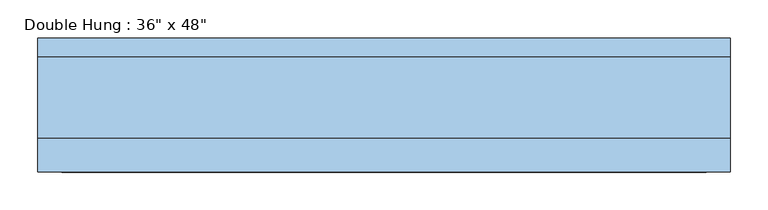
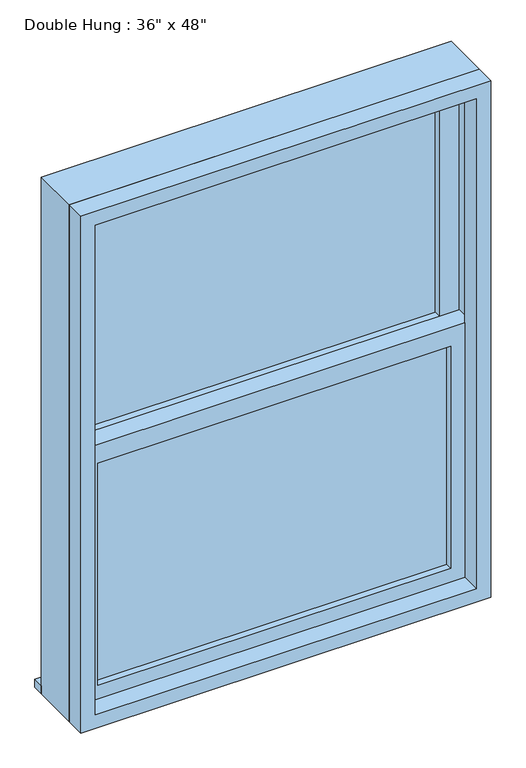
"""IFC4 building model written with IfcOpenShell, lengths in millimetres: window geometry."""

from ifc_helpers import new_model, si_unit, frame, origin, place, context, project, spatial, polyline, outline, extrude, source, transform, mapped, element, save


def window_d6fe7540(model_context):
    return source(origin(), model_context, "Body", "SweptSolid", [
        extrude(outline(polyline([(-393.7, -3.175), (393.7, -3.175), (393.7, -15.875), (-393.7, -15.875), (-393.7, -3.175)])), frame((0.0, 0.0, 977.9), z_axis=(0.0, 0.0, 1.0), x_axis=(1.0, 0.0, 0.0)), (0.0, 0.0, 1.0), 523.875),
        extrude(outline(polyline([(1546.225, -438.15), (933.45, -438.15), (933.45, 438.15), (1546.225, 438.15), (1546.225, -438.15)]), holes=[polyline([(1501.775, -393.7), (1501.775, 393.7), (977.9, 393.7), (977.9, -393.7), (1501.775, -393.7)])]), frame((0.0, -31.75, 0.0), z_axis=(0.0, 1.0, 0.0), x_axis=(0.0, 0.0, 1.0)), (0.0, 0.0, 1.0), 44.45),
        extrude(outline(polyline([(-457.2, 101.6), (457.2, 101.6), (457.2, 76.2), (-457.2, 76.2), (-457.2, 101.6)])), frame((0.0, 0.0, 914.4), z_axis=(0.0, 0.0, 1.0), x_axis=(1.0, 0.0, 0.0)), (0.0, 0.0, 1.0), 19.05),
        extrude(outline(polyline([(393.7, 28.575), (-393.7, 28.575), (-393.7, 41.275), (393.7, 41.275), (393.7, 28.575)])), frame((0.0, 0.0, 1546.225), z_axis=(0.0, 0.0, 1.0), x_axis=(1.0, 0.0, 0.0)), (0.0, 0.0, 1.0), 523.875),
        extrude(outline(polyline([(2114.55, -438.15), (1501.775, -438.15), (1501.775, 438.15), (2114.55, 438.15), (2114.55, -438.15)]), holes=[polyline([(2070.1, -393.7), (2070.1, 393.7), (1546.225, 393.7), (1546.225, -393.7), (2070.1, -393.7)])]), frame((0.0, 12.7, 0.0), z_axis=(0.0, 1.0, 0.0), x_axis=(0.0, 0.0, 1.0)), (0.0, 0.0, 1.0), 44.45),
        extrude(outline(polyline([(2133.6, -457.2), (914.4, -457.2), (914.4, 457.2), (2133.6, 457.2), (2133.6, -457.2)]), holes=[polyline([(2101.85, -425.45), (2101.85, 425.45), (946.15, 425.45), (946.15, -425.45), (2101.85, -425.45)])]), frame((0.0, -76.2, 0.0), z_axis=(0.0, 1.0, 0.0), x_axis=(0.0, 0.0, 1.0)), (0.0, 0.0, 1.0), 44.45),
        extrude(outline(polyline([(2133.6, 457.2), (2133.6, -457.2), (914.4, -457.2), (914.4, 457.2), (2133.6, 457.2)]), holes=[polyline([(2114.55, 438.15), (933.45, 438.15), (933.45, -438.15), (2114.55, -438.15), (2114.55, 438.15)])]), frame((0.0, -31.75, 0.0), z_axis=(0.0, 1.0, 0.0), x_axis=(0.0, 0.0, 1.0)), (0.0, 0.0, 1.0), 107.95),
    ])


if __name__ == "__main__":
    model = new_model("IFC4")
    model_context = context("Model", 3, world=origin())
    ifc_project = project(units=[si_unit("LENGTHUNIT", "METRE", prefix="MILLI")], contexts=[model_context])
    site = spatial("IfcSite", under=ifc_project)
    building = spatial("IfcBuilding", under=site)
    placement = place(None, origin())
    window_shape = window_d6fe7540(model_context)
    element("IfcWindow", 1, ObjectType="Double Hung : 36\" x 48\"", at=placement, inside=building, context=model_context, shape_type="MappedRepresentation", body=[
        mapped(window_shape, transform((0.0, 0.0, 0.0), x_axis=(1.0, 0.0, 0.0), y_axis=(0.0, 1.0, 0.0), z_axis=(0.0, 0.0, 1.0))),
    ])
    save(model, "model.ifc")

# Revit data of these elements
# Type "Double Hung : 36\" x 48\""
#   Type Mark = "26"
#   Construction Type Id = "GSP4R"
#   Assembly Code = "B2020100"
#   Analytic Construction = "1/8 in Pilkington single glazing"
#   Visual Light Transmittance = 0.9
#   Solar Heat Gain Coefficient = 0.78
#   Heat Transfer Coefficient (U) = 0.6496 BTU/(h·ft²·°F)
#   Height = 4' - 0"
#   Default Sill Height = 3' - 0"
#   Width = 3' - 0"
#   Window Inset = 0' - 0 3/4"
#   Define Thermal Properties by = 1
#   Glass Pane Material = Glass
#   Sash Material = Sash
#   Description = (empty or 0)
#   Wall Closure = (empty or 0)
# Element 1 (IfcWindow, "Double Hung : 36\" x 48\"")
#   Materials on its faces: "Sash", "Glass"
# Materials
#   "Glass": class "Glass", colour RGB 0 128 192, transparency 0.75, Description = "Soda Lime Glass", Cost = 0
#   "Sash": class "Wood", colour RGB 224 178 126, transparency 0
